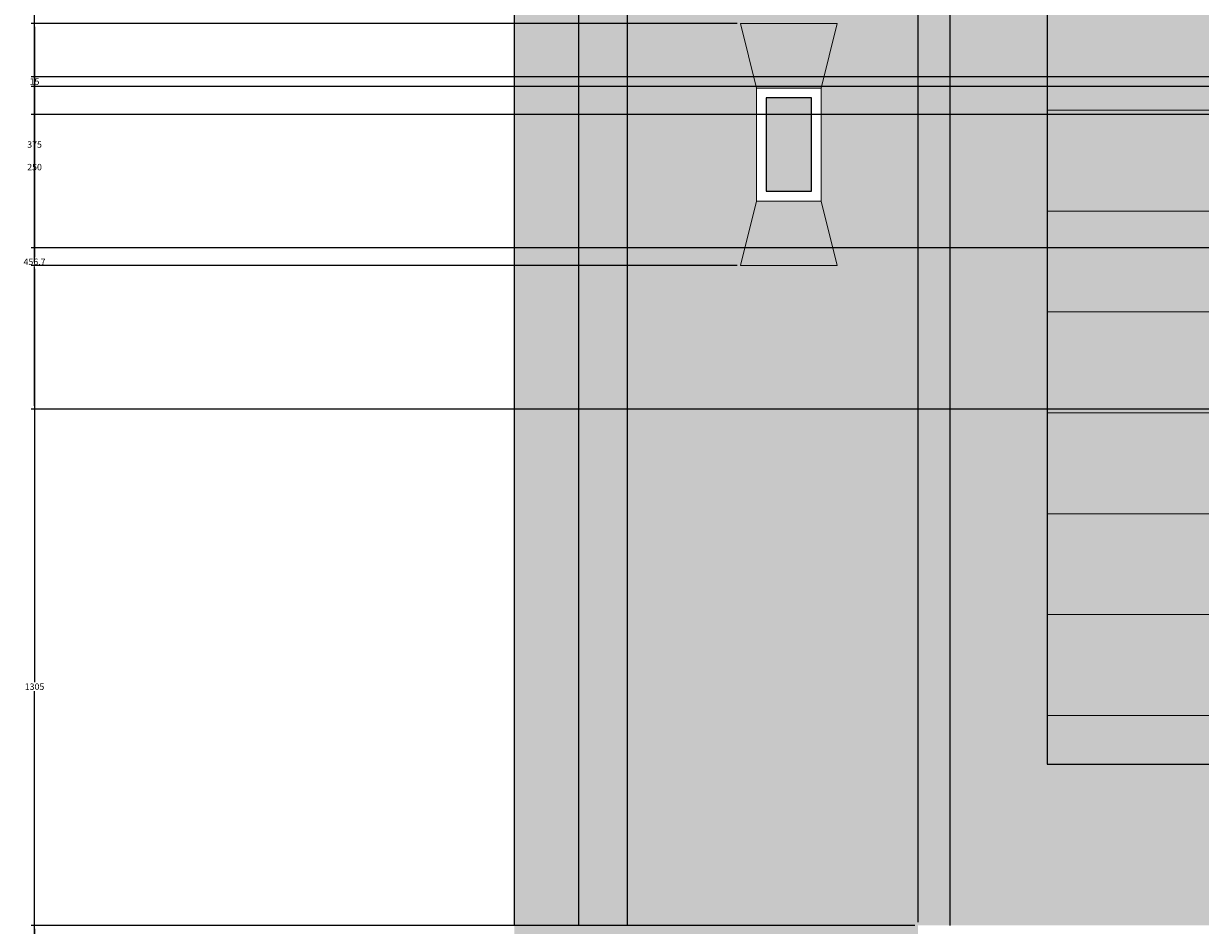
# Model space of a CAD drawing. Units: millimetres. Extents: x 2970 to 7764, y 2196 to 7505.
# Tile 6 of 13: x 2970 to 4793, y 4206 to 5603. Entities that reach past the tile are written whole.
import ezdxf

# ---------------------------------------------------------------- set-up
doc = ezdxf.new("R2010")
doc.units = ezdxf.units.MM
doc.header["$MEASUREMENT"] = 0
for name, color, linetype, lineweight in [('A-ANNO-DIMS', 2, 'Continuous', 18), ('A-ELEV', 7, 'Continuous', 25), ('A-ELEV-PATT', 8, 'Continuous', 13), ('E-LITE', 2, 'Continuous', 18)]:
    doc.layers.add(name, color=color, linetype=linetype, lineweight=lineweight)
doc.styles.get("Standard").update_dxf_attribs({"font": 'arial.ttf'})
doc.dimstyles.get("Standard").update_dxf_attribs({"dimtxt": 10, "dimasz": 5, "dimexe": 5, "dimexo": 5, "dimgap": 2, "dimtad": 0, "dimtih": 1, "dimtoh": 1, "dimdec": 0, "dimzin": 0, "dimdsep": 46, "dimtxsty": 'Standard', "dimcen": 2, "dimadec": 0, "dimazin": 0, "dimtfac": 1, "dimtdec": 0, "dimtofl": 0, "dimtmove": 0, "dimatfit": 3, "dimfxl": 1, "dimtolj": 1, "dimtzin": 0, "dimarcsym": 0})

# ---------------------------------------------------------------- blocks, each defined once
blk = doc.blocks.new('WALL-SCONCE')
for p, q in [((4105.5, 5503.3), (4080.5, 5603.3)), ((4080.5, 5603.3), (4230.5, 5603.3)), ((4205.5, 5503.3), (4230.5, 5603.3)), ((4080.5, 5228.3), (4105.5, 5328.3)), ((4230.5, 5228.3), (4205.5, 5328.3)), ((4080.5, 5228.3), (4230.5, 5228.3))]:
    blk.add_line(p, q)
blk.add_lwpolyline([(4105.5, 5328.3), (4205.5, 5328.3), (4205.5, 5503.3), (4105.5, 5503.3)], close=True)
blk = doc.blocks.new('*D23')
at = {"layer": 'A-ANNO-DIMS', "color": 0, "lineweight": -2, "transparency": 16777216}
for p, q in [((4075.5, 5228.3), (2982.5, 5228.3)), ((2987.5, 5223.3), (2987.5, 4582.9)), ((2987.5, 3928.3), (2987.5, 4568.7)), ((4075.5, 3923.3), (2982.5, 3923.3))]:
    blk.add_line(p, q, dxfattribs=at)
at = {"layer": 'A-ANNO-DIMS', "color": 0, "transparency": 16777216}
for points in [[(2986.7, 5223.3), (2988.3, 5223.3), (2987.5, 5228.3)], [(2986.7, 3928.3), (2988.3, 3928.3), (2987.5, 3923.3)]]:
    blk.add_solid(points, dxfattribs=at)
at = {"layer": 'Defpoints', "color": 0, "transparency": 16777216}
for p in [(2987.5, 5228.3), (4080.5, 5228.3), (4080.5, 3923.3)]:
    blk.add_point(p, dxfattribs=at)
at = {"layer": 'A-ANNO-DIMS', "color": 0, "transparency": 16777216, "insert": (2987.5, 4575.8), "char_height": 10, "attachment_point": 5}
blk.add_mtext('\\A1;1305', dxfattribs=at)
blk = doc.blocks.new('*D24')
at = {"layer": 'A-ANNO-DIMS', "color": 0, "lineweight": -2, "transparency": 16777216}
for p, q in [((4075.5, 5603.3), (2982.5, 5603.3)), ((2987.5, 5598.3), (2987.5, 5422.9)), ((2987.5, 5233.3), (2987.5, 5408.7)), ((4075.5, 5228.3), (2982.5, 5228.3))]:
    blk.add_line(p, q, dxfattribs=at)
at = {"layer": 'A-ANNO-DIMS', "color": 0, "transparency": 16777216}
for points in [[(2986.7, 5598.3), (2988.3, 5598.3), (2987.5, 5603.3)], [(2986.7, 5233.3), (2988.3, 5233.3), (2987.5, 5228.3)]]:
    blk.add_solid(points, dxfattribs=at)
at = {"layer": 'Defpoints', "color": 0, "transparency": 16777216}
for p in [(2987.5, 5603.3), (4080.5, 5603.3), (4080.5, 5228.3)]:
    blk.add_point(p, dxfattribs=at)
at = {"layer": 'A-ANNO-DIMS', "color": 0, "transparency": 16777216, "insert": (2987.5, 5415.8), "char_height": 10, "attachment_point": 5}
blk.add_mtext('\\A1;375', dxfattribs=at)
blk = doc.blocks.new('*D34')
at = {"layer": 'A-ANNO-DIMS', "color": 0, "lineweight": -2, "transparency": 16777216}
for p, q in [((4355.5, 4210.8), (4355.5, 7503.8)), ((4360.5, 7498.8), (4607.5, 7498.8)), ((4880.5, 7498.8), (4633.5, 7498.8)), ((4885.5, 4210.8), (4885.5, 7503.8))]:
    blk.add_line(p, q, dxfattribs=at)
at = {"layer": 'A-ANNO-DIMS', "color": 0, "transparency": 16777216}
for points in [[(4360.5, 7499.6), (4360.5, 7498), (4355.5, 7498.8)], [(4880.5, 7499.6), (4880.5, 7498), (4885.5, 7498.8)]]:
    blk.add_solid(points, dxfattribs=at)
at = {"layer": 'Defpoints', "color": 0, "transparency": 16777216}
for p in [(4885.5, 7498.8), (4355.5, 4205.8), (4885.5, 4205.8)]:
    blk.add_point(p, dxfattribs=at)
at = {"layer": 'A-ANNO-DIMS', "color": 0, "transparency": 16777216, "insert": (4620.5, 7498.8), "char_height": 10, "attachment_point": 5}
blk.add_mtext('\\A1;530', dxfattribs=at)
blk = doc.blocks.new('*D46')
at = {"layer": 'A-ANNO-DIMS', "color": 0, "lineweight": -2, "transparency": 16777216}
for p, q in [((4350.5, 4205.8), (2982.5, 4205.8)), ((2987.5, 4200.8), (2987.5, 3912.9)), ((2987.5, 3610.8), (2987.5, 3898.7)), ((4880.5, 3605.8), (2982.5, 3605.8))]:
    blk.add_line(p, q, dxfattribs=at)
at = {"layer": 'A-ANNO-DIMS', "color": 0, "transparency": 16777216}
for points in [[(2986.7, 4200.8), (2988.3, 4200.8), (2987.5, 4205.8)], [(2986.7, 3610.8), (2988.3, 3610.8), (2987.5, 3605.8)]]:
    blk.add_solid(points, dxfattribs=at)
at = {"layer": 'Defpoints', "color": 0, "transparency": 16777216}
for p in [(2987.5, 4205.8), (4355.5, 4205.8), (4885.5, 3605.8)]:
    blk.add_point(p, dxfattribs=at)
at = {"layer": 'A-ANNO-DIMS', "color": 0, "transparency": 16777216, "insert": (2987.5, 3905.8), "char_height": 10, "attachment_point": 5}
blk.add_mtext('\\A1;600', dxfattribs=at)
blk = doc.blocks.new('*D61')
at = {"layer": 'A-ANNO-DIMS', "color": 0, "lineweight": -2, "transparency": 16777216}
for p, q in [((5010.8, 5462.5), (2982.5, 5462.5)), ((2987.5, 5457.5), (2987.5, 5241.2)), ((2987.5, 5010.8), (2987.5, 5227)), ((5750.5, 5005.8), (2982.5, 5005.8))]:
    blk.add_line(p, q, dxfattribs=at)
at = {"layer": 'A-ANNO-DIMS', "color": 0, "transparency": 16777216}
for points in [[(2986.7, 5457.5), (2988.3, 5457.5), (2987.5, 5462.5)], [(2986.7, 5010.8), (2988.3, 5010.8), (2987.5, 5005.8)]]:
    blk.add_solid(points, dxfattribs=at)
at = {"layer": 'Defpoints', "color": 0, "transparency": 16777216}
for p in [(5015.8, 5462.5), (2987.5, 5005.8), (5755.5, 5005.8)]:
    blk.add_point(p, dxfattribs=at)
at = {"layer": 'A-ANNO-DIMS', "color": 0, "transparency": 16777216, "insert": (2987.5, 5234.1), "char_height": 10, "attachment_point": 5}
blk.add_mtext('\\A1;456.7', dxfattribs=at)
blk = doc.blocks.new('*D76')
at = {"layer": 'A-ANNO-DIMS', "color": 0, "lineweight": -2, "transparency": 16777216}
for p, q in [((6100.5, 6055.8), (2982.5, 6055.8)), ((2987.5, 6050.8), (2987.5, 5662.9)), ((2987.5, 5260.8), (2987.5, 5648.7)), ((6100.5, 5255.8), (2982.5, 5255.8))]:
    blk.add_line(p, q, dxfattribs=at)
at = {"layer": 'A-ANNO-DIMS', "color": 0, "transparency": 16777216}
for points in [[(2986.7, 6050.8), (2988.3, 6050.8), (2987.5, 6055.8)], [(2986.7, 5260.8), (2988.3, 5260.8), (2987.5, 5255.8)]]:
    blk.add_solid(points, dxfattribs=at)
at = {"layer": 'Defpoints', "color": 0, "transparency": 16777216}
for p in [(2987.5, 6055.8), (6105.5, 6055.8), (6105.5, 5255.8)]:
    blk.add_point(p, dxfattribs=at)
at = {"layer": 'A-ANNO-DIMS', "color": 0, "transparency": 16777216, "insert": (2987.5, 5655.8), "char_height": 10, "attachment_point": 5}
blk.add_mtext('\\A1;800', dxfattribs=at)
blk = doc.blocks.new('*D79')
at = {"layer": 'A-ANNO-DIMS', "color": 0, "lineweight": -2, "transparency": 16777216}
for p, q in [((6000.5, 5505.8), (2982.5, 5505.8)), ((2987.5, 5500.8), (2987.5, 5387.9)), ((2987.5, 5260.8), (2987.5, 5373.7)), ((6000.5, 5255.8), (2982.5, 5255.8))]:
    blk.add_line(p, q, dxfattribs=at)
at = {"layer": 'A-ANNO-DIMS', "color": 0, "transparency": 16777216}
for points in [[(2986.7, 5500.8), (2988.3, 5500.8), (2987.5, 5505.8)], [(2986.7, 5260.8), (2988.3, 5260.8), (2987.5, 5255.8)]]:
    blk.add_solid(points, dxfattribs=at)
at = {"layer": 'Defpoints', "color": 0, "transparency": 16777216}
for p in [(2987.5, 5505.8), (6005.5, 5505.8), (6005.5, 5255.8)]:
    blk.add_point(p, dxfattribs=at)
at = {"layer": 'A-ANNO-DIMS', "color": 0, "transparency": 16777216, "insert": (2987.5, 5380.8), "char_height": 10, "attachment_point": 5}
blk.add_mtext('\\A1;250', dxfattribs=at)
blk = doc.blocks.new('*D80')
at = {"layer": 'A-ANNO-DIMS', "color": 0, "lineweight": -2, "transparency": 16777216}
for p, q in [((2987.5, 5525.8), (2987.5, 5530.8)), ((6000.5, 5520.8), (2982.5, 5520.8)), ((6000.5, 5505.8), (2982.5, 5505.8)), ((2987.5, 5500.8), (2987.5, 5495.8))]:
    blk.add_line(p, q, dxfattribs=at)
at = {"layer": 'A-ANNO-DIMS', "color": 0, "transparency": 16777216}
for points in [[(2986.7, 5525.8), (2988.3, 5525.8), (2987.5, 5520.8)], [(2986.7, 5500.8), (2988.3, 5500.8), (2987.5, 5505.8)]]:
    blk.add_solid(points, dxfattribs=at)
at = {"layer": 'Defpoints', "color": 0, "transparency": 16777216}
for p in [(2987.5, 5520.8), (6005.5, 5520.8), (6005.5, 5505.8)]:
    blk.add_point(p, dxfattribs=at)
at = {"layer": 'A-ANNO-DIMS', "color": 0, "transparency": 16777216, "insert": (2987.5, 5513.3), "char_height": 10, "attachment_point": 5}
blk.add_mtext('\\A1;15', dxfattribs=at)

msp = doc.modelspace()

# ---------------------------------------------------------------- hatches: boundary and pattern name
at = {"layer": 'A-ELEV-PATT'}
h = msp.add_hatch(color=256, dxfattribs=at)
h.dxf.hatch_style = 1
h.paths.add_polyline_path([(6405.5, 7255.789), (4305.5, 7255.789), (4305.5, 6505.789), (3730.5, 6505.789), (3730.5, 4205.789), (3730.5, 2945.789), (3730.5, 2895.789), (3830.5, 2895.789), (3830.5, 4205.789), (3830.5, 6405.789), (4405.5, 6405.789), (4405.5, 4205.789), (6905.5, 4205.789), (6905.5, 2945.789), (6905.5, 2845.789), (7155.5, 2845.789), (7155.5, 2945.789), (7155.5, 4205.789), (7155.5, 4455.789), (4555.5, 4455.789), (4555.5, 6505.789), (4555.5, 7005.789), (6155.5, 7005.789), (6155.5, 6755.789), (6405.5, 6755.789)])
h.paths.add_polyline_path([(7405.5, 6755.789), (6155.5, 6755.789), (5755.5, 6755.789), (5755.5, 5005.789), (7405.5, 5005.789)])
h.paths.add_polyline_path([(7155.5, 6505.789), (7155.5, 5255.789), (6005.5, 5255.789), (6005.5, 6505.789)], flags=16)
h.paths.add_polyline_path([(6105.5, 5520.789), (6105.5, 6055.789), (6455.5, 6055.789), (6455.5, 5520.789), (6655.5, 5520.789), (6655.5, 5605.789), (6655.5, 5955.789), (6955.5, 5955.789), (6955.5, 5605.789), (6955.5, 5520.789)], flags=0)
h.paths.add_polyline_path([(6425.5, 5755.789), (6425.5, 5655.789), (6425.5, 5555.789), (6405.5, 5555.789), (6405.5, 5755.789)], flags=0)
h.paths.add_polyline_path([(6955.5, 5505.789), (6955.5, 5405.789), (6655.5, 5405.789), (6655.5, 5505.789)], flags=0)
h = msp.add_hatch(color=256, dxfattribs=at)
h.set_gradient(color1=(147, 149, 152), color2=(199, 200, 202), name='CURVED')
h.paths.add_polyline_path([(6955.5, 4455.789), (6955.5, 5005.789), (5755.5, 5005.789), (5755.5, 6755.789), (6155.5, 6755.789), (6155.5, 7005.789), (4555.5, 7005.789), (4555.5, 6505.789), (4555.5, 4455.789)])
h.paths.add_polyline_path([(5015.81, 5462.49), (5015.81, 6062.49), (5455.81, 6062.49), (5455.81, 5462.49)], flags=16)
h.paths.add_polyline_path([(5035.81, 5482.49), (5035.81, 6042.49), (5155.81, 6042.49), (5155.81, 5482.49)], flags=0)
h.paths.add_polyline_path([(5175.81, 5482.49), (5175.81, 6042.49), (5295.81, 6042.49), (5295.81, 5482.49)], flags=0)
h.paths.add_polyline_path([(5315.81, 5482.49), (5315.81, 6042.49), (5435.81, 6042.49), (5435.81, 5482.49)], flags=0)
h.paths.add_polyline_path([(4865.81, 6162.49), (4865.81, 6212.49), (4840.81, 6212.49), (4840.81, 6237.49), (5630.81, 6237.49), (5630.81, 6212.49), (5605.81, 6212.49), (5605.81, 6162.49), (5015.81, 6162.49)], flags=16)
h = msp.add_hatch(dxfattribs=at)
h.set_pattern_fill('ANSI31', color=256, scale=1250, angle=135, style=0)
h.paths.add_polyline_path([(5755.5, 6755.789), (6155.5, 6755.789), (6155.5, 7005.789), (4555.5, 7005.789), (4555.5, 6505.789), (4555.5, 4455.789), (6955.5, 4455.789), (6955.5, 5005.789), (5755.5, 5005.789)])
h.paths.add_polyline_path([(5015.81, 5462.49), (5015.81, 6062.49), (5455.81, 6062.49), (5455.81, 5462.49)], flags=16)
h.paths.add_polyline_path([(5035.81, 5482.49), (5035.81, 6042.49), (5155.81, 6042.49), (5155.81, 5482.49)], flags=0)
h.paths.add_polyline_path([(5175.81, 5482.49), (5175.81, 6042.49), (5295.81, 6042.49), (5295.81, 5482.49)], flags=0)
h.paths.add_polyline_path([(5315.81, 5482.49), (5315.81, 6042.49), (5435.81, 6042.49), (5435.81, 5482.49)], flags=0)
h.paths.add_polyline_path([(4865.81, 6162.49), (4865.81, 6212.49), (4840.81, 6212.49), (4840.81, 6237.49), (5630.81, 6237.49), (5630.81, 6212.49), (5605.81, 6212.49), (5605.81, 6162.49), (5015.81, 6162.49)], flags=16)
h = msp.add_hatch(color=256, dxfattribs=at)
h.set_gradient(color1=(76, 38, 38), color2=(99, 100, 102), name='INVSPHERICAL')
h.paths.add_polyline_path([(3830.5, 6405.789), (3830.5, 4205.789), (3830.5, 2895.789), (3905.5, 2895.789), (3905.5, 4205.789), (3905.5, 6255.789), (4405.5, 6255.789), (4405.5, 6405.789)])
h = msp.add_hatch(color=256, dxfattribs=at)
h.set_gradient(color1=(53, 53, 54), color2=(99, 100, 102), name='SPHERICAL')
h.paths.add_polyline_path([(4405.5, 6255.789), (3905.5, 6255.789), (3905.5, 4205.789), (3905.5, 2895.789), (4355.5, 2895.789), (4355.5, 2995.799, -0.50803883), (4340.162, 3038.75, -0.52056705), (4337.177, 3086.472, -0.19797947), (4355.5, 3108.072), (4355.5, 4205.789), (4405.5, 4205.789)])
h.paths.add_polyline_path([(4080.5, 5228.289), (4105.5, 5328.289), (4105.5, 5503.289), (4080.5, 5603.289), (4230.5, 5603.289), (4205.5, 5503.289), (4205.5, 5328.289), (4230.5, 5228.289)], flags=16)
h.paths.add_polyline_path([(4120.5, 5343.289), (4120.5, 5488.289), (4190.5, 5488.289), (4190.5, 5343.289)], flags=0)
h.paths.add_polyline_path([(4230.5, 3923.289), (4205.5, 3823.289), (4205.5, 3648.289), (4230.5, 3548.289), (4080.5, 3548.289), (4105.5, 3648.289), (4105.5, 3823.289), (4080.5, 3923.289)], flags=16)
h.paths.add_polyline_path([(4190.5, 3808.289), (4190.5, 3663.289), (4120.5, 3663.289), (4120.5, 3808.289)], flags=0)
h = msp.add_hatch(color=256, dxfattribs=at)
h.set_gradient(color1=(241, 235, 31), color2=(99, 100, 102), name='INVCURVED')
h.paths.add_polyline_path([(4105.5, 5503.289), (4205.5, 5503.289), (4230.5, 5603.289), (4080.5, 5603.289)])
h = msp.add_hatch(color=256, dxfattribs=at)
h.set_gradient(color1=(248, 215, 49), color2=(241, 235, 31), name='INVCYLINDER')
h.paths.add_polyline_path([(5490.5, 3733.289), (5560.5, 3733.289), (5560.5, 3878.289), (5490.5, 3878.289)])
h.paths.add_polyline_path([(4720.5, 3878.289), (4650.5, 3878.289), (4650.5, 3733.289), (4720.5, 3733.289)])
h.paths.add_polyline_path([(4120.5, 3663.289), (4190.5, 3663.289), (4190.5, 3808.289), (4120.5, 3808.289)])
h.paths.add_polyline_path([(4190.5, 5488.289), (4120.5, 5488.289), (4120.5, 5343.289), (4190.5, 5343.289)])
h = msp.add_hatch(color=256, dxfattribs=at)
h.set_gradient(color1=(241, 235, 31), color2=(99, 100, 102), name='CURVED')
h.paths.add_polyline_path([(4230.5, 5228.289), (4205.5, 5328.289), (4105.5, 5328.289), (4080.5, 5228.289)])

# ---------------------------------------------------------------- linework, layer by layer
at = {"layer": 'A-ELEV'}
for p, q in [((3730.5, 4205.789), (3730.5, 6505.789)), ((4555.5, 6505.789), (4555.5, 4455.789)), ((3830.5, 4205.789), (3830.5, 6405.789)), ((4405.5, 4205.789), (4405.5, 6405.789)), ((3905.5, 4205.789), (3905.5, 6255.789)), ((4555.5, 4455.789), (7155.5, 4455.789))]:
    msp.add_line(p, q, dxfattribs=at)
msp.add_lwpolyline([(4120.5, 5343.289), (4190.5, 5343.289), (4190.5, 5488.289), (4120.5, 5488.289)], close=True, dxfattribs=at)

# ---------------------------------------------------------------- block references
at = {"layer": 'E-LITE'}
msp.add_blockref('WALL-SCONCE', (0, 0), dxfattribs=at)

# ---------------------------------------------------------------- dimensions: what is measured, and where the dimension line sits
at = {"layer": 'A-ANNO-DIMS'}
dim = msp.add_linear_dim(base=(4885.5, 7498.789), p1=(4355.5, 4205.789), p2=(4885.5, 4205.789), dimstyle='Standard', override={"dimdec": 0, "dimlfac": 1, "dimrnd": 0, "dimzin": 0, "dimdsep": 46, "dimlunit": 2}, dxfattribs=at)
dim.commit()
dim.dimension.update_dxf_attribs({"geometry": '*D34', "text_midpoint": (4620.5, 7498.789)})
for base, p1, p2, override, picture, middle in [((2987.5, 6055.789), (6105.5, 5255.789), (6105.5, 6055.789), {"dimdec": 0, "dimlfac": 1, "dimrnd": 0, "dimzin": 0, "dimdsep": 46, "dimlunit": 2}, '*D76', (2987.5, 5655.789)), ((2987.5, 5603.289), (4080.5, 5228.289), (4080.5, 5603.289), {"dimdec": 0, "dimlfac": 1, "dimrnd": 0, "dimzin": 0, "dimdsep": 46, "dimlunit": 2}, '*D24', (2987.5, 5415.789)), ((2987.5, 5520.789), (6005.5, 5505.789), (6005.5, 5520.789), {"dimdec": 0, "dimlfac": 1, "dimrnd": 0, "dimzin": 0, "dimdsep": 46, "dimlunit": 2}, '*D80', (2987.5, 5513.289)), ((2987.5, 5505.789), (6005.5, 5255.789), (6005.5, 5505.789), {"dimdec": 0, "dimlfac": 1, "dimrnd": 0, "dimzin": 0, "dimdsep": 46, "dimlunit": 2}, '*D79', (2987.5, 5380.789)), ((2987.5, 5005.789), (5015.81, 5462.49), (5755.5, 5005.789), {"dimdec": 1, "dimlfac": 1, "dimrnd": 0, "dimzin": 0, "dimdsep": 46, "dimlunit": 2}, '*D61', (2987.5, 5234.139)), ((2987.5, 5228.289), (4080.5, 3923.289), (4080.5, 5228.289), {"dimdec": 0, "dimlfac": 1, "dimrnd": 0, "dimzin": 0, "dimdsep": 46, "dimlunit": 2}, '*D23', (2987.5, 4575.789)), ((2987.5, 4205.789), (4885.5, 3605.789), (4355.5, 4205.789), {"dimdec": 0, "dimlfac": 1, "dimrnd": 0, "dimzin": 0, "dimdsep": 46, "dimlunit": 2}, '*D46', (2987.5, 3905.789))]:
    dim = msp.add_linear_dim(base=base, p1=p1, p2=p2, angle=90, dimstyle='Standard', override=override, dxfattribs=at)
    dim.commit()
    dim.dimension.update_dxf_attribs({"geometry": picture, "text_midpoint": middle})

doc.saveas('drawing.dxf')
